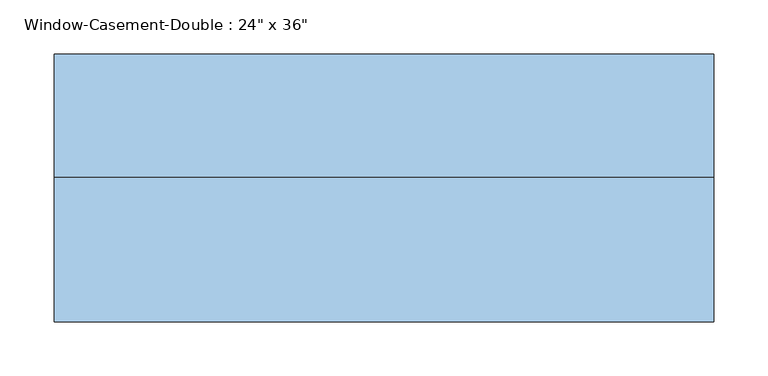
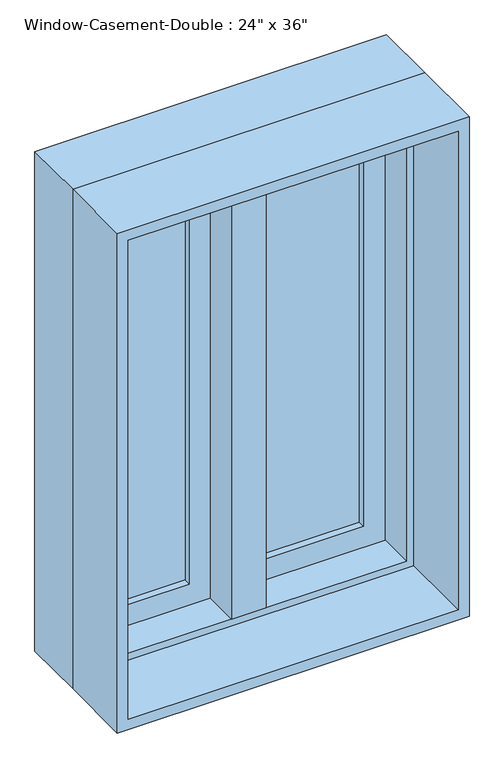
"""IFC4 building model written with IfcOpenShell, lengths in millimetres: window geometry."""

from ifc_helpers import new_model, si_unit, frame, origin, place, context, project, spatial, polyline, outline, extrude, faceted_brep, source, transform, mapped, element, save


def window_c417fced(model_context):
    return source(origin(), model_context, "Body", "SolidModel", [
        faceted_brep([(9.525, 133.35, 1816.1), (-9.525, 133.35, 1816.1), (-9.525, 82.55, 1816.1), (9.525, 82.55, 1816.1), (9.525, 133.35, 927.1), (9.525, 82.55, 927.1), (-9.525, 82.55, 927.1), (-9.525, 133.35, 927.1), (-9.525, 82.55, 946.15), (-9.525, 82.55, 1797.05), (-30.1625, 82.55, 946.15), (-30.1625, 82.55, 1797.05), (-30.1625, 19.05, 946.15), (-30.1625, 19.05, 1797.05), (30.1625, 19.05, 946.15), (30.1625, 19.05, 1797.05), (30.1625, 82.55, 946.15), (30.1625, 82.55, 1797.05), (9.525, 82.55, 946.15), (9.525, 82.55, 1797.05)], [[[0, 1, 2, 3]], [[4, 5, 6, 7]], [[1, 0, 4, 7]], [[2, 1, 7, 6, 8, 9]], [[9, 8, 10, 11]], [[11, 10, 12, 13]], [[13, 12, 14, 15]], [[15, 14, 16, 17]], [[17, 16, 18, 19]], [[0, 3, 19, 18, 5, 4]], [[18, 8, 6, 5]], [[9, 19, 3, 2]], [[8, 18, 16, 14, 12, 10]], [[19, 9, 11, 13, 15, 17]]]),
        extrude(outline(polyline([(-66.675, 114.3), (-66.675, 107.95), (-234.95, 107.95), (-234.95, 114.3), (-66.675, 114.3)])), frame((0.0, 0.0, 984.25), z_axis=(0.0, 0.0, 1.0), x_axis=(1.0, 0.0, 0.0)), (0.0, 0.0, 1.0), 774.7),
        extrude(outline(polyline([(-234.95, 95.25), (-234.95, 101.6), (-66.675, 101.6), (-66.675, 95.25), (-234.95, 95.25)])), frame((0.0, 0.0, 984.25), z_axis=(0.0, 0.0, 1.0), x_axis=(1.0, 0.0, 0.0)), (0.0, 0.0, 1.0), 774.7),
        extrude(outline(polyline([(234.95, 114.3), (234.95, 107.95), (66.675, 107.95), (66.675, 114.3), (234.95, 114.3)])), frame((0.0, 0.0, 984.25), z_axis=(0.0, 0.0, 1.0), x_axis=(1.0, 0.0, 0.0)), (0.0, 0.0, 1.0), 774.7),
        extrude(outline(polyline([(66.675, 95.25), (66.675, 101.6), (234.95, 101.6), (234.95, 95.25), (66.675, 95.25)])), frame((0.0, 0.0, 984.25), z_axis=(0.0, 0.0, 1.0), x_axis=(1.0, 0.0, 0.0)), (0.0, 0.0, 1.0), 774.7),
        extrude(outline(polyline([(1816.1, -292.1), (927.1, -292.1), (927.1, -9.525), (1816.1, -9.525), (1816.1, -292.1)]), holes=[polyline([(1758.95, -66.675), (984.25, -66.675), (984.25, -234.95), (1758.95, -234.95), (1758.95, -66.675)])]), frame((0.0, 82.55, 0.0), z_axis=(0.0, 1.0, 0.0), x_axis=(0.0, 0.0, 1.0)), (0.0, 0.0, 1.0), 44.45),
        extrude(outline(polyline([(927.1, 292.1), (1816.1, 292.1), (1816.1, 9.525), (927.1, 9.525), (927.1, 292.1)]), holes=[polyline([(984.25, 66.675), (1758.95, 66.675), (1758.95, 234.95), (984.25, 234.95), (984.25, 66.675)])]), frame((0.0, 82.55, 0.0), z_axis=(0.0, 1.0, 0.0), x_axis=(0.0, 0.0, 1.0)), (0.0, 0.0, 1.0), 44.45),
        extrude(outline(polyline([(1828.8, -304.8), (914.4, -304.8), (914.4, 304.8), (1828.8, 304.8), (1828.8, -304.8)]), holes=[polyline([(1809.75, 285.75), (933.45, 285.75), (933.45, -285.75), (1809.75, -285.75), (1809.75, 285.75)])]), frame((0.0, -114.3, 0.0), z_axis=(0.0, 1.0, 0.0), x_axis=(0.0, 0.0, 1.0)), (0.0, 0.0, 1.0), 133.35),
        faceted_brep([(273.05, 82.55, 1797.05), (273.05, 19.05, 1797.05), (-273.05, 19.05, 1797.05), (-273.05, 82.55, 1797.05), (292.1, 133.35, 1816.1), (292.1, 82.55, 1816.1), (-292.1, 82.55, 1816.1), (-292.1, 133.35, 1816.1), (304.8, 19.05, 1828.8), (304.8, 133.35, 1828.8), (-304.8, 133.35, 1828.8), (-304.8, 19.05, 1828.8), (-273.05, 19.05, 946.15), (-273.05, 82.55, 946.15), (-292.1, 82.55, 927.1), (-292.1, 133.35, 927.1), (-304.8, 133.35, 914.4), (-304.8, 19.05, 914.4), (273.05, 19.05, 946.15), (273.05, 82.55, 946.15), (292.1, 82.55, 927.1), (292.1, 133.35, 927.1), (304.8, 133.35, 914.4), (304.8, 19.05, 914.4)], [[[0, 1, 2, 3]], [[4, 5, 6, 7]], [[8, 9, 10, 11]], [[3, 2, 12, 13]], [[7, 6, 14, 15]], [[11, 10, 16, 17]], [[13, 12, 18, 19]], [[15, 14, 20, 21]], [[17, 16, 22, 23]], [[11, 17, 23, 8], [1, 18, 12, 2]], [[19, 18, 1, 0]], [[5, 20, 14, 6], [3, 13, 19, 0]], [[21, 20, 5, 4]], [[23, 22, 9, 8]], [[9, 22, 16, 10], [7, 15, 21, 4]]]),
    ])


if __name__ == "__main__":
    model = new_model("IFC4")
    model_context = context("Model", 3, world=origin())
    ifc_project = project(units=[si_unit("LENGTHUNIT", "METRE", prefix="MILLI")], contexts=[model_context])
    site = spatial("IfcSite", under=ifc_project)
    building = spatial("IfcBuilding", under=site)
    placement = place(None, origin())
    window_shape = window_c417fced(model_context)
    element("IfcWindow", 1, ObjectType="Window-Casement-Double : 24\" x 36\"", at=placement, inside=building, context=model_context, shape_type="MappedRepresentation", body=[
        mapped(window_shape, transform((0.0, 0.0, 0.0), x_axis=(1.0, 0.0, 0.0), y_axis=(0.0, 1.0, 0.0), z_axis=(0.0, 0.0, 1.0))),
    ])
    save(model, "model.ifc")

# Revit data of these elements
# Type "Window-Casement-Double : 24\" x 36\""
#   Type Mark = "14"
#   Fire Rating = "0.5h"
#   Assembly Code = "B2020100"
#   Analytic Construction = "Double glazing - domestic"
#   Frame Extension [instance default] = 0' - 0 1/4"
#   Window Inset [instance default] = 0' - 0"
#   Wall Thickness [instance default] = 0' - 6"
#   Interior Wall Closure [instance default] = 0' - 2 1/4"
#   Half Width = 1' - 0"
#   Visual Light Transmittance = 0.81
#   Thermal Resistance (R) = 1.8146 (h·ft²·°F)/BTU
#   Solar Heat Gain Coefficient = 0.76
#   Rough Width = 2' - 0 1/2"
#   Rough Height = 3' - 0 1/2"
#   Height = 3' - 0"
#   Heat Transfer Coefficient (U) = 0.5511 BTU/(h·ft²·°F)
#   Exterior Wall Closure [instance default] = 0' - 1 1/4"
#   Extension Jamb [instance default] = 0' - 2 1/4"
#   Default Sill Height = 3' - 0"
#   Width = 2' - 0"
#   Define Thermal Properties by = 0
#   Muntin Visibility = yes
#   Interior Trim Visibility [instance default] = yes
#   Exterior Trim Visibility [instance default] = yes
#   Extension Jamb Visibility [instance default] = yes
#   Interior Trim Material = Wood - Stained
#   Muntin Pattern = Muntin Pattern_2x2 : Muntin Pattern_2x2
#   Interior Trim = Trim-Window-Interior-Flat : Picture Frame
#   Interior Frame Material = Wood - Stained
#   Glass Panel Material = Glass
#   Exterior Trim Material = Clad - White
#   Exterior Trim = Trim-Window-Exterior-Flat : with Sill
#   Exterior Frame Material = Clad - White
#   Wall Closure = (empty or 0)
# Element 1 (IfcWindow, "Window-Casement-Double : 24\" x 36\"")
#   Wall Thickness = 0' - 9"
#   Extension Jamb = 0' - 5 1/4"
#   Materials on its faces: "Wood - Stained", "Glass", "Clad - White"
# Materials
#   "Wood - Stained": class "Wood", colour RGB 224 178 126, transparency 0, Cost = 0
#   "Glass": class "Glass", colour RGB 0 128 192, transparency 0.75, Description = "Soda Lime Glass", Cost = 0
#   "Clad - White": class "Wood", colour RGB 242 242 238, transparency 0, Cost = 0
